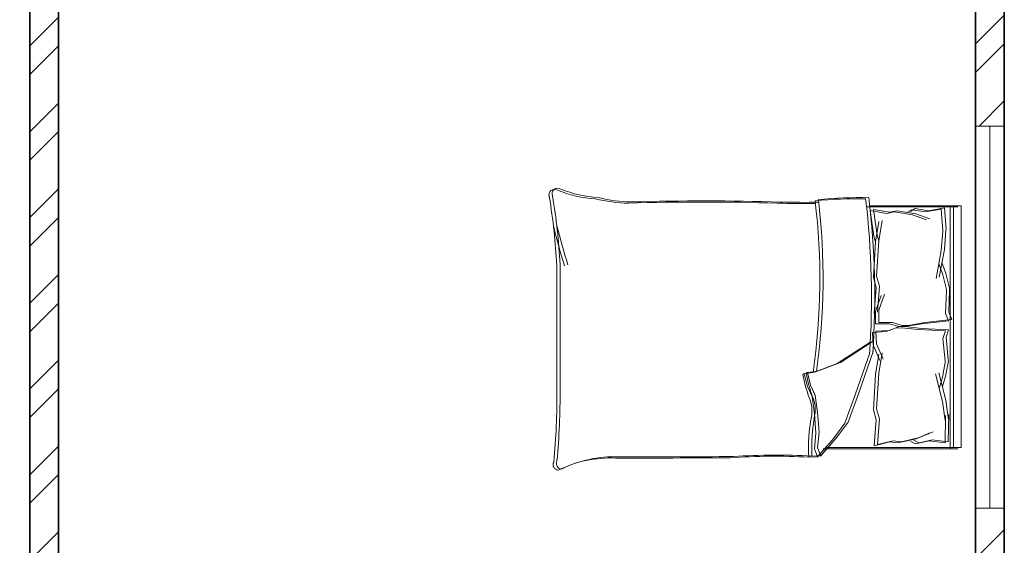
# Model space of a CAD drawing. Units: inches. Extents: x 1962 to 2771, y 1245 to 2660.
# Tile 13 of 114: x 2506 to 2661, y 1527 to 1609. Entities that reach past the tile are written whole.
import ezdxf

# ---------------------------------------------------------------- set-up
doc = ezdxf.new("R2010")
doc.units = ezdxf.units.IN
for name, color, linetype, lineweight in [('A-FURN', 8, 'Continuous', 13), ('A-GLAZ', 4, 'Continuous', 18), ('A-WALL', 7, 'Continuous', 35), ('A-WALL-PATT', 252, 'Continuous', 13)]:
    doc.layers.add(name, color=color, linetype=linetype, lineweight=lineweight)

# ---------------------------------------------------------------- blocks, each defined once
blk = doc.blocks.new('BED-PLAN')
for p, q in [((22.05, 42.03), (19.47, 39.08)), ((22.05, 42.02), (19.47, 39.08)), ((22.56, 42.21), (19.98, 39.26)), ((22.56, 42.21), (19.98, 39.26)), ((23.44, 42.09), (22.05, 42.03, 3.08)), ((23.44, 42.09), (22.05, 42.02, 3.08)), ((22.55, 40.8), (22.05, 42.03)), ((22.55, 40.8), (22.05, 42.02)), ((23.95, 42.27), (22.56, 42.21, 3.08)), ((23.95, 42.27), (22.56, 42.21, 3.08)), ((23.06, 40.98), (22.56, 42.21)), ((23.06, 40.98), (22.56, 42.21)), ((0, 40.75), (21.15, 40.75)), ((0, 40.75), (21.15, 40.75)), ((0, 2.76), (0, 40.75)), ((0.51, 40.93), (21.66, 40.93)), ((0.51, 40.93), (21.66, 40.93)), ((1.22, 2.76), (1.22, 40.75)), ((1.22, 2.76), (1.22, 40.75)), ((1.73, 2.95), (1.73, 40.93)), ((1.73, 2.95), (1.73, 40.93)), ((13.17, 40.3), (10.68, 39.68)), ((13.17, 40.3), (10.68, 39.68)), ((13.68, 40.48), (11.19, 39.87)), ((13.68, 40.48), (11.19, 39.87)), ((12.85, 36.22), (13.17, 40.3)), ((12.85, 36.22), (13.17, 40.3)), ((13.36, 36.4), (13.68, 40.48)), ((13.36, 36.4), (13.68, 40.48)), ((22.3, 38.34), (22.55, 40.8)), ((22.3, 38.34), (22.55, 40.8)), ((22.81, 38.52), (23.06, 40.98)), ((22.81, 38.52), (23.06, 40.98)), ((2.03, 39.83), (1.96, 35.54)), ((2.03, 39.83), (1.96, 35.54)), ((2.03, 39.83), (4.58, 39.53)), ((2.03, 39.83), (4.58, 39.53)), ((2.54, 40.02), (2.46, 35.72)), ((2.54, 40.02), (2.46, 35.72)), ((2.54, 40.02), (5.09, 39.72)), ((2.54, 40.02), (5.09, 39.72)), ((6.56, 39.2), (4.43, 38.26)), ((6.56, 39.2), (4.43, 38.26)), ((4.58, 39.53), (6.63, 40.01)), ((4.58, 39.53), (6.63, 40.01)), ((7.07, 39.38), (4.94, 38.44)), ((7.07, 39.38), (4.94, 38.44)), ((5.09, 39.72), (7.14, 40.19)), ((5.09, 39.72), (7.14, 40.19)), ((9.4, 39.83), (6.56, 39.2)), ((9.4, 39.83), (6.56, 39.2)), ((6.63, 40.01), (7.46, 39.6)), ((6.63, 40.01), (7.46, 39.6)), ((9.91, 40.02), (7.07, 39.38)), ((9.91, 40.02), (7.07, 39.38)), ((7.14, 40.19), (7.97, 39.78)), ((7.14, 40.19), (7.97, 39.78)), ((10.68, 39.68), (9.4, 39.83)), ((10.68, 39.68), (9.4, 39.83)), ((11.19, 39.87), (9.91, 40.02)), ((11.19, 39.87), (9.91, 40.02)), ((19.47, 39.08), (17.75, 36.74)), ((19.47, 39.08), (17.75, 36.74)), ((19.98, 39.26), (18.26, 36.92)), ((19.98, 39.26), (18.26, 36.92)), ((22.55, 35.26), (22.3, 38.34)), ((22.55, 35.26), (22.3, 38.34)), ((23.06, 35.45), (22.81, 38.52)), ((23.06, 35.44), (22.81, 38.52)), ((1.96, 35.54), (2.02, 36.34)), ((1.96, 35.54), (2.02, 36.34)), ((2.02, 36.34), (2.44, 33.32)), ((2.02, 36.34), (2.44, 33.32)), ((2.46, 35.72), (2.53, 36.52)), ((2.46, 35.72), (2.53, 36.52)), ((2.53, 36.52), (2.95, 33.5)), ((2.53, 36.52), (2.95, 33.5)), ((13.3, 34.66), (12.85, 36.22)), ((13.3, 34.66), (12.85, 36.22)), ((13.8, 34.84), (13.36, 36.4)), ((13.8, 34.84), (13.36, 36.4)), ((17.75, 36.74), (16.15, 32.31)), ((17.75, 36.74), (16.15, 32.31)), ((18.26, 36.92), (16.66, 32.49)), ((18.26, 36.92), (16.66, 32.49)), ((12.95, 29.09), (13.3, 34.66)), ((12.95, 29.09), (13.3, 34.66)), ((13.46, 29.27), (13.8, 34.84)), ((13.46, 29.27), (13.8, 34.84)), ((22.92, 32.56), (22.55, 35.26)), ((22.92, 32.55), (22.55, 35.26)), ((23.42, 32.74), (23.06, 35.45)), ((23.42, 32.74), (23.06, 35.44)), ((2.44, 33.32), (3.52, 29.01)), ((2.44, 33.32), (3.52, 29.01)), ((2.95, 33.5), (4.02, 29.19)), ((2.95, 33.5), (4.02, 29.19)), ((16.66, 32.49), (14.33, 25.86)), ((16.66, 32.49), (14.33, 25.86)), ((23.65, 30.95), (22.92, 32.56)), ((23.65, 30.95), (22.92, 32.55)), ((24.16, 31.14), (23.42, 32.74)), ((24.16, 31.14), (23.42, 32.74)), ((2.92, 31.16), (2.45, 29.52)), ((2.92, 31.16), (2.45, 29.52)), ((3.43, 31.34), (2.96, 29.7)), ((3.43, 31.34), (2.96, 29.7)), ((16.15, 32.31), (13.82, 25.68)), ((16.15, 32.31), (13.82, 25.68)), ((24.15, 28.99), (23.65, 30.95)), ((24.15, 28.98), (23.65, 30.95)), ((24.65, 29.17), (24.16, 31.14)), ((24.65, 29.17), (24.16, 31.14)), ((62.99, 11.98), (62.99, 31.54)), ((62.99, 11.97), (62.99, 31.54)), ((63.5, 12.16), (63.5, 31.72)), ((63.5, 12.16), (63.5, 31.72)), ((2.45, 29.52), (2.02, 27.19)), ((2.45, 29.52), (2.02, 27.19)), ((2.96, 29.7), (2.52, 27.37)), ((2.96, 29.7), (2.52, 27.37)), ((12.42, 25.89), (12.95, 29.09)), ((12.42, 25.89), (12.95, 29.09)), ((12.93, 26.07), (13.46, 29.27)), ((12.93, 26.07), (13.46, 29.27)), ((18.98, 27.38), (22.55, 28.74)), ((18.98, 27.38), (22.55, 28.74)), ((19.49, 27.57), (23.06, 28.92)), ((19.49, 27.57), (23.06, 28.92)), ((22.55, 28.74), (24.15, 28.99)), ((22.55, 28.74), (24.15, 28.98)), ((23.06, 28.92), (24.65, 29.17)), ((23.06, 28.92), (24.65, 29.17)), ((2.02, 27.19), (2.03, 26.94)), ((2.02, 27.19), (2.03, 26.93)), ((2.03, 26.94), (2.37, 23.42)), ((2.03, 26.93), (2.37, 23.42)), ((2.52, 27.37), (2.54, 27.12)), ((2.52, 27.37), (2.54, 27.12)), ((2.54, 27.12), (2.88, 23.6)), ((2.54, 27.12), (2.88, 23.6)), ((13.31, 24.44), (12.28, 26.89)), ((13.31, 24.44), (12.28, 26.88)), ((13.81, 24.63), (12.79, 27.07)), ((13.81, 24.63), (12.79, 27.07)), ((13.82, 24.05), (18.98, 27.38)), ((13.82, 24.05), (18.98, 27.38)), ((14.33, 24.24), (19.49, 27.57)), ((14.33, 24.24), (19.49, 27.57)), ((2.37, 23.42), (1.98, 22.24)), ((2.37, 23.42), (1.98, 22.24)), ((2.88, 23.6), (2.49, 22.42)), ((2.88, 23.6), (2.49, 22.42)), ((13.43, 22.49), (13.31, 24.44)), ((13.43, 22.49), (13.31, 24.44)), ((13.94, 22.68), (13.81, 24.63)), ((13.94, 22.68), (13.81, 24.63)), ((1.98, 22.24), (6.25, 22.05)), ((1.98, 22.24), (6.25, 22.05)), ((2.49, 22.42), (6.76, 22.23)), ((2.49, 22.42), (6.76, 22.23)), ((6.25, 22.05), (8.81, 21.75)), ((6.25, 22.05), (8.81, 21.75)), ((6.25, 21.3), (8.78, 21.76)), ((6.25, 21.3), (8.78, 21.76)), ((6.76, 22.23), (9.31, 21.93)), ((6.76, 22.23), (9.31, 21.93)), ((8.78, 21.76), (9.81, 21.76)), ((8.78, 21.76), (9.81, 21.76)), ((8.81, 21.75), (9.84, 21.81)), ((8.81, 21.75), (9.84, 21.81)), ((9.31, 21.93), (10.35, 21.99)), ((9.31, 21.93), (10.35, 21.99)), ((9.81, 21.76), (11.3, 21.3)), ((9.81, 21.76), (11.3, 21.3)), ((9.84, 21.81), (11.3, 22.36)), ((9.84, 21.81), (11.3, 22.36)), ((10.35, 21.99), (11.81, 22.54)), ((10.35, 21.99), (11.81, 22.54)), ((11.3, 22.36), (13.43, 22.49)), ((11.3, 22.36), (13.43, 22.49)), ((11.81, 22.54), (13.94, 22.68)), ((11.81, 22.54), (13.94, 22.68)), ((1.49, 20.65), (5.74, 21.11)), ((1.49, 20.65), (5.74, 21.11)), ((1.95, 19.51), (1.49, 20.65)), ((1.95, 19.51), (1.49, 20.65)), ((1.99, 20.84), (6.25, 21.3)), ((1.99, 20.84), (6.25, 21.3)), ((2.45, 19.69), (1.99, 20.84)), ((2.45, 19.69), (1.99, 20.84)), ((5.74, 21.11), (8.27, 21.57)), ((5.74, 21.11), (8.27, 21.57)), ((8.27, 21.57), (9.3, 21.57)), ((8.27, 21.57), (9.3, 21.57)), ((9.3, 21.57), (10.8, 21.11)), ((9.3, 21.57), (10.8, 21.11)), ((10.8, 21.11), (12.93, 21.11)), ((10.8, 21.11), (12.93, 21.11)), ((11.3, 21.3), (13.44, 21.3)), ((11.3, 21.3), (13.44, 21.3)), ((12.93, 21.11), (12.93, 19.16)), ((12.93, 21.11), (12.93, 19.16)), ((13.44, 21.3), (13.44, 19.34)), ((13.44, 21.3), (13.44, 19.34)), ((1.83, 15.97), (1.95, 19.51)), ((1.83, 15.97), (1.95, 19.51)), ((2.34, 16.15), (2.45, 19.69)), ((2.34, 16.15), (2.45, 19.69)), ((12.93, 19.16), (12.06, 16.66)), ((12.93, 19.16), (12.06, 16.66)), ((13.44, 19.34), (12.57, 16.84)), ((13.44, 19.34), (12.57, 16.84)), ((12.85, 15.41), (13.17, 19.49)), ((12.85, 15.41), (13.17, 19.49)), ((13.36, 15.59), (13.68, 19.67)), ((13.36, 15.59), (13.68, 19.67)), ((1.83, 15.72), (1.83, 15.97)), ((1.83, 15.72), (1.83, 15.97)), ((2.41, 13.42), (1.83, 15.72)), ((2.41, 13.42), (1.83, 15.72)), ((2.34, 15.9), (2.34, 16.15)), ((2.34, 15.9), (2.34, 16.15)), ((2.91, 13.6), (2.34, 15.9)), ((2.91, 13.6), (2.34, 15.9)), ((13.8, 14.03), (13.36, 15.59)), ((13.8, 14.03), (13.36, 15.59)), ((2.64, 9.63), (3.44, 13.99)), ((2.64, 9.63), (3.44, 13.99)), ((3.14, 9.81), (3.95, 14.17)), ((3.14, 9.81), (3.95, 14.17)), ((13.3, 13.85), (12.85, 15.41)), ((13.3, 13.85), (12.85, 15.41)), ((13.46, 8.46), (13.8, 14.03)), ((13.46, 8.46), (13.8, 14.03)), ((2.98, 11.81), (2.41, 13.42)), ((2.98, 11.81), (2.41, 13.42)), ((3.49, 11.99), (2.91, 13.6)), ((3.49, 11.99), (2.91, 13.6)), ((12.95, 8.28), (13.3, 13.85)), ((12.95, 8.28), (13.3, 13.85)), ((2.41, 6.59), (2.64, 9.63)), ((2.41, 6.59), (2.64, 9.63)), ((2.91, 6.77), (3.14, 9.81)), ((2.91, 6.77), (3.14, 9.81)), ((12.42, 5.07), (12.95, 8.28)), ((12.42, 5.07), (12.95, 8.28)), ((12.93, 5.26), (13.46, 8.46)), ((12.93, 5.26), (13.46, 8.46)), ((12.95, 8.28), (13.21, 7.38)), ((12.95, 8.28), (13.21, 7.38)), ((13.46, 8.46), (13.72, 7.56)), ((13.46, 8.46), (13.72, 7.56)), ((2.39, 6.5), (2.41, 6.59)), ((2.39, 6.5), (2.41, 6.59)), ((2.65, 3.1), (2.39, 6.5)), ((2.65, 3.1), (2.39, 6.5)), ((2.9, 6.68), (2.91, 6.77)), ((2.9, 6.68), (2.91, 6.77)), ((3.16, 3.28), (2.9, 6.68)), ((3.16, 3.28), (2.9, 6.68)), ((13.21, 7.38), (13.78, 3.33)), ((13.21, 7.38), (13.78, 3.33)), ((13.72, 7.56), (14.29, 3.51)), ((13.72, 7.56), (14.29, 3.51)), ((7.12, 4.02), (4.93, 4.82)), ((7.12, 4.02), (4.93, 4.82)), ((7.63, 4.2), (5.44, 5)), ((7.63, 4.2), (5.44, 5)), ((2.64, 3.1), (5.16, 3.56)), ((2.64, 3.1), (5.16, 3.56)), ((3.14, 3.28), (5.67, 3.74)), ((3.14, 3.28), (5.67, 3.74)), ((5.16, 3.56), (7.23, 3.21)), ((5.16, 3.56), (7.23, 3.21)), ((5.67, 3.74), (7.74, 3.39)), ((5.67, 3.74), (7.74, 3.39)), ((9.99, 3.56), (7.12, 4.02)), ((9.99, 3.56), (7.12, 4.02)), ((7.23, 3.21), (8.04, 3.67)), ((7.23, 3.21), (8.04, 3.67)), ((10.5, 3.74), (7.63, 4.2)), ((10.5, 3.74), (7.63, 4.2)), ((7.74, 3.39), (8.55, 3.85)), ((7.74, 3.39), (8.55, 3.85)), ((11.26, 3.79), (9.99, 3.56)), ((11.26, 3.79), (9.99, 3.56)), ((11.76, 3.97), (10.5, 3.74)), ((11.76, 3.97), (10.5, 3.74)), ((13.78, 3.33), (11.26, 3.79)), ((13.78, 3.33), (11.26, 3.79)), ((14.29, 3.51), (11.76, 3.97)), ((14.29, 3.51), (11.76, 3.97)), ((14.4, 2.76), (0, 2.76)), ((14.4, 2.76), (0, 2.76)), ((14.9, 2.95), (0.51, 2.95)), ((14.9, 2.95), (0.51, 2.95))]:
    blk.add_line(p, q)
for centre, radius, start, end in [((54.58, 60.54), 18.33, 267.4714, 296.4681), ((54.58, 60.54), 18.33, 267.4714, 296.4681), ((55.09, 60.72), 18.33, 267.4714, 296.4681), ((55.09, 60.72), 18.33, 267.4714, 296.4681), ((62.69, 43.25), 0.876, 332.6588, 86.02), ((62.69, 43.25), 0.876, 332.6588, 86.02), ((63.2, 43.43), 0.876, 332.6588, 86.02), ((63.2, 43.43), 0.876, 332.6588, 86.02), ((-5.29, 40.8), 28.76, 349.8763, 2.5657), ((-5.29, 40.8), 28.76, 349.8763, 2.5657), ((28.87, 144.88), 102.94, 266.9791, 273.8365), ((28.87, 144.88), 102.94, 266.9791, 273.8365), ((-4.78, 40.98), 28.76, 349.8763, 2.5657), ((-4.78, 40.98), 28.76, 349.8763, 2.5657), ((29.37, 145.06), 102.94, 266.9791, 273.8365), ((29.37, 145.06), 102.94, 266.9791, 273.8365), ((53.91, -3583.94), 3626.16, 90.00217, 90.28689), ((53.91, -3583.94), 3626.16, 90.00217, 90.28689), ((54.42, -3583.75), 3626.16, 90.00217, 90.28689), ((54.42, -3583.75), 3626.16, 90.00217, 90.28689), ((168.74, 32.71), 105.75, 174.4998, 180.6351), ((168.74, 32.71), 105.75, 174.4998, 180.6351), ((169.24, 32.89), 105.75, 174.4998, 180.6351), ((169.24, 32.89), 105.75, 174.4998, 180.6351), ((27.87, 34.77), 4.95, 168.6608, 203.7384), ((27.87, 34.77), 4.95, 168.6608, 203.7384), ((28.38, 34.95), 4.95, 168.6608, 203.7384), ((28.38, 34.95), 4.95, 168.6608, 203.7384), ((1.18, 24.77), 23.57, 10.6617, 19.8806), ((1.18, 24.76), 23.57, 10.6617, 19.8806), ((1.69, 24.95), 23.57, 10.6617, 19.8806), ((1.69, 24.95), 23.57, 10.6617, 19.8806), ((124.25, 14.12), 102.56, 171.7845, 186.9006), ((124.25, 14.11), 102.56, 171.7845, 186.9006), ((124.76, 14.3), 102.56, 171.7845, 186.9006), ((124.76, 14.3), 102.56, 171.7845, 186.9006), ((24.2, 29.12), 0.147, 250.2464, 1.1377), ((24.2, 29.12), 0.147, 250.2464, 1.1377), ((24.7, 29.3), 0.147, 250.2464, 1.1377), ((24.7, 29.3), 0.147, 250.2464, 1.1377), ((144.71, 16.98), 131.13, 176.0865, 186.7821), ((144.71, 16.98), 131.13, 176.0865, 186.7821), ((145.22, 17.16), 131.13, 176.0865, 186.7821), ((145.22, 17.16), 131.13, 176.0865, 186.7821), ((-18.85, -13.69), 84.62, 13.3832, 17.7053), ((-18.85, -13.69), 84.62, 13.3832, 17.7053), ((-18.34, -13.51), 84.62, 13.3832, 17.7053), ((-18.34, -13.51), 84.62, 13.3832, 17.7053), ((159.64, 17.03), 96.78, 182.9958, 189.4091), ((159.64, 17.03), 96.78, 182.9958, 189.4091), ((160.15, 17.21), 96.78, 182.9958, 189.4091), ((160.15, 17.21), 96.78, 182.9958, 189.4091), ((15.97, 67.7), 66.22, 268.7218, 275.604), ((15.97, 67.7), 66.22, 268.7218, 275.604), ((16.48, 67.88), 66.22, 268.7218, 275.604), ((16.48, 67.88), 66.22, 268.7218, 275.604), ((24.78, -132.99), 135.22, 88.4762, 91.0082), ((24.78, -132.99), 135.22, 88.4762, 91.0082), ((25.29, -132.81), 135.22, 88.4762, 91.0082), ((25.29, -132.81), 135.22, 88.4762, 91.0082), ((40.23, 385.38), 383.38, 268.2277, 271.7185), ((40.23, 385.38), 383.38, 268.2277, 271.7185), ((40.74, 385.56), 383.38, 268.2277, 271.7185), ((40.74, 385.56), 383.38, 268.2277, 271.7185), ((51.28, -21.38), 23.56, 76.0648, 88.9113), ((51.28, -21.38), 23.56, 76.0648, 88.9113), ((51.79, -21.2), 23.56, 76.0648, 88.9113), ((51.79, -21.2), 23.56, 76.0648, 88.9113), ((56.37, -17.03), 18.73, 67.9751, 86.652), ((56.37, -17.03), 18.73, 67.9751, 86.652), ((55.86, -17.22), 18.73, 67.9751, 86.652), ((55.86, -17.22), 18.73, 67.9751, 86.652), ((63.37, 0.87), 0.866, 236.1736, 23.4781), ((63.37, 0.87), 0.866, 236.1736, 23.4781), ((63.87, 1.05), 0.866, 236.1736, 23.4781), ((63.87, 1.05), 0.866, 236.1736, 23.4781)]:
    blk.add_arc(centre, radius, start, end)
blk = doc.blocks.new('WIN-60IN-A')
for p, q in [((0, 60), (4.5, 60)), ((4.5, 60), (2.25, 60)), ((2.25, 60), (2.25, 0)), ((2.25, 0), (0, 0)), ((0, 0), (4.5, 0))]:
    blk.add_line(p, q)

msp = doc.modelspace()

# ---------------------------------------------------------------- hatches: boundary and pattern name
at = {"layer": 'A-WALL-PATT'}
h = msp.add_hatch(dxfattribs=at)
h.set_pattern_fill('ANSI32', color=256)
h.paths.add_polyline_path([(2090.8074, 2467.3437), (2141.6481, 2467.3437), (2141.6481, 2469.5937), (2141.6481, 2471.8437), (2086.3074, 2471.8437), (2086.3074, 2422.5333), (2090.8074, 2422.5333)])
h.paths.add_polyline_path([(2282.7664, 2471.8437), (2204.8982, 2471.8437), (2204.8982, 2467.3437), (2234.8074, 2467.3437), (2234.8074, 2311.3437), (2228.7492, 2311.3437), (2228.7492, 2306.8437), (2234.8074, 2306.8437), (2331.9227, 2306.8437), (2331.9227, 2309.0937), (2331.9227, 2311.3437), (2239.3074, 2311.3437), (2239.3074, 2467.3437), (2282.7664, 2467.3437), (2282.7664, 2469.5937)])
h.paths.add_polyline_path([(2471.4531, 2519.8437), (2552.011, 2519.8437), (2564.3996, 2519.8437), (2564.3996, 2511.1389), (2568.8996, 2511.1389), (2568.8996, 2524.3437), (2466.9531, 2524.3437), (2466.9531, 2471.8437), (2450.0749, 2471.8437), (2446.4672, 2471.8437), (2446.4672, 2467.3437), (2450.0749, 2467.3437), (2475.9988, 2467.3437), (2475.9988, 2469.5937), (2475.9988, 2471.8437), (2471.4531, 2471.8437)])
h.paths.add_polyline_path([(2575.2231, 2469.5937), (2575.2231, 2471.8437), (2568.8996, 2471.8437), (2568.8996, 2487.1389), (2564.3996, 2487.1389), (2564.3996, 2471.8437), (2556.511, 2471.8437), (2499.2904, 2471.8437), (2499.2904, 2467.3437), (2507.8074, 2467.3437), (2507.8074, 2311.3437), (2414.863, 2311.3437), (2414.863, 2306.8437), (2512.3074, 2306.8437), (2517.0114, 2306.8437), (2517.0114, 2309.0937), (2517.0114, 2311.3437), (2512.3074, 2311.3437), (2512.3074, 2467.3437), (2575.2231, 2467.3437)])
h.paths.add_polyline_path([(2660.8074, 2471.8437), (2600.9602, 2471.8437), (2600.9602, 2467.3437), (2656.3074, 2467.3437), (2656.3074, 2432.5704), (2660.8074, 2432.5704)])
h.paths.add_polyline_path([(2660.8074, 2372.5704), (2656.3074, 2372.5704), (2656.3074, 2311.3437), (2600.276, 2311.3437), (2600.276, 2309.0937), (2600.276, 2306.8437), (2656.3074, 2306.8437), (2656.3074, 2296.2593), (2660.8074, 2296.2593)])
h.paths.add_polyline_path([(2572.3074, 2306.8437), (2577.1385, 2306.8437), (2577.1385, 2311.3437), (2551.082, 2311.3437), (2551.082, 2306.8437), (2567.8074, 2306.8437), (2567.8074, 2258.8437), (2540.0574, 2258.8437), (2540.0574, 2256.5937), (2540.0574, 2254.3437), (2567.8074, 2254.3437), (2656.3074, 2254.3437), (2656.3074, 2236.9085), (2660.8074, 2236.9085), (2660.8074, 2272.2593), (2656.3074, 2272.2593), (2656.3074, 2258.8437), (2572.3074, 2258.8437)])
h.paths.add_polyline_path([(2512.3074, 2254.3437), (2518.8716, 2254.3437), (2518.8716, 2256.5937), (2518.8716, 2258.8437), (2507.8074, 2258.8437), (2507.8074, 2177.8437), (2567.8074, 2177.8437), (2567.8074, 2172.9628), (2572.3074, 2172.9628), (2572.3074, 2177.8437), (2656.3074, 2177.8437), (2656.3074, 2166.4846), (2660.8074, 2166.4846), (2660.8074, 2200.9085), (2656.3074, 2200.9085), (2656.3074, 2182.3437), (2512.3074, 2182.3437)])
h.paths.add_polyline_path([(2656.3074, 2129.8437), (2572.3074, 2129.8437), (2572.3074, 2150.3044), (2570.0574, 2150.3044), (2567.8074, 2150.3044), (2567.8074, 2129.8437), (2507.8074, 2129.8437), (2507.8074, 2116.3027), (2510.0574, 2116.3027), (2512.3074, 2116.3027), (2512.3074, 2125.3437), (2567.8074, 2125.3437), (2572.3074, 2125.3437), (2656.3074, 2125.3437)])
h.paths.add_polyline_path([(2090.8074, 2362.5333), (2086.3074, 2362.5333), (2086.3074, 2298.6242), (2090.8074, 2298.6242), (2090.8074, 2306.8437), (2174.8074, 2306.8437), (2174.8074, 2286.4178), (2179.3074, 2286.4178), (2179.3074, 2306.8437), (2192.8641, 2306.8437), (2192.8641, 2309.0937), (2192.8641, 2311.3437), (2090.8074, 2311.3437)])
h.paths.add_polyline_path([(2209.156, 2258.8437), (2179.3074, 2258.8437), (2179.3074, 2263.2236), (2177.0574, 2263.2236), (2174.8074, 2263.2236), (2174.8074, 2258.8437), (2090.8074, 2258.8437), (2090.8074, 2274.6242), (2086.3074, 2274.6242), (2086.3074, 2238.2967), (2088.5574, 2238.2967), (2090.8074, 2238.2967), (2090.8074, 2254.3437), (2209.156, 2254.3437)])
h.paths.add_polyline_path([(2090.8074, 2177.8437), (2234.8074, 2177.8437), (2234.8074, 2173.1428), (2239.3074, 2173.1428), (2239.3074, 2258.8437), (2230.8442, 2258.8437), (2230.8442, 2256.5937), (2230.8442, 2254.3437), (2234.8074, 2254.3437), (2234.8074, 2182.3437), (2090.8074, 2182.3437), (2090.8074, 2202.2967), (2086.3074, 2202.2967), (2086.3074, 2140.0389), (2090.8074, 2140.0389)])
h.paths.add_polyline_path([(2090.8074, 2080.0389), (2086.3074, 2080.0389), (2086.3074, 2033.8437), (2090.8074, 2033.8437)], flags=17)
h.paths.add_polyline_path([(2244.9405, 2033.8437), (2239.3074, 2033.8437), (2239.3074, 2142.0665), (2237.2592, 2142.0665), (2234.8074, 2142.0665), (2234.8074, 2033.8437), (2090.8074, 2033.8437), (2076.5204, 2033.8437), (2072.0204, 2033.8437), (2072.0204, 2000.4493), (2076.5204, 2000.4493), (2076.5204, 2029.3437), (2090.8074, 2029.3437), (2244.9405, 2029.3437), (2244.9405, 2031.5937)])
h.paths.add_polyline_path([(2234.8074, 1933.3437), (2076.5204, 1933.3437), (2076.5204, 1952.4493), (2074.2704, 1952.4493), (2072.0204, 1952.4493), (2072.0204, 1933.3437), (2072.0204, 1928.8437), (2234.8074, 1928.8437)])
h.paths.add_polyline_path([(2090.8074, 1928.8437), (2086.3074, 1928.8437), (2086.3074, 1906.5013), (2090.8074, 1906.5013)])
h.paths.add_polyline_path([(2090.8074, 1846.5013), (2086.3074, 1846.5013), (2086.3074, 1769.9917), (2088.5574, 1769.9917), (2090.8074, 1769.9917), (2090.8074, 1780.3437), (2234.8074, 1780.3437), (2234.8074, 1708.3437), (2230.3764, 1708.3437), (2230.3764, 1703.8437), (2239.3074, 1703.8437), (2239.3074, 1792.6669), (2237.0574, 1792.6669), (2234.8074, 1792.6669), (2234.8074, 1784.8437), (2090.8074, 1784.8437)])
h.paths.add_polyline_path([(2239.3074, 1928.8437), (2244.9405, 1928.8437), (2244.9405, 1931.0937), (2244.9405, 1933.3437), (2234.8074, 1933.3437), (2234.8074, 1928.8437), (2234.8074, 1825.5949), (2239.3074, 1825.5949)])
h.paths.add_polyline_path([(2148.0425, 1649.0937), (2148.0425, 1651.3437), (2090.8074, 1651.3437), (2090.8074, 1646.8437), (2148.0425, 1646.8437)], flags=0)
h.paths.add_polyline_path([(2207.5601, 1708.3437), (2090.8074, 1708.3437), (2090.8074, 1703.8437), (2174.8074, 1703.8437), (2174.8074, 1651.3437), (2170.4457, 1651.3437), (2170.4457, 1646.8437), (2195.9924, 1646.8437), (2195.9924, 1649.0937), (2195.9924, 1651.3437), (2179.3074, 1651.3437), (2179.3074, 1703.8437), (2207.5601, 1703.8437), (2207.5601, 1706.0937)])
h.paths.add_polyline_path([(2090.8074, 1733.9917), (2086.3074, 1733.9917), (2086.3074, 1696.1032), (2088.5574, 1696.1032), (2090.8074, 1696.1032)])
h.paths.add_polyline_path([(2090.8074, 1672.1032), (2086.3074, 1672.1032), (2086.3074, 1600.3335), (2090.8074, 1600.3335)])
h.paths.add_polyline_path([(2090.8074, 1540.3335), (2086.3074, 1540.3335), (2086.3074, 1486.3437), (2139.6766, 1486.3437), (2139.6766, 1490.8437), (2090.8074, 1490.8437)])
h.paths.add_polyline_path([(2302.3876, 1490.8437), (2239.3074, 1490.8437), (2239.3074, 1646.8437), (2335.9994, 1646.8437), (2335.9994, 1651.3437), (2229.884, 1651.3437), (2229.884, 1646.8437), (2234.8074, 1646.8437), (2234.8074, 1490.8437), (2202.7103, 1490.8437), (2202.7103, 1488.5937), (2202.7103, 1486.3437), (2275.0699, 1486.3437), (2275.0699, 1475.772), (2279.5699, 1475.772), (2279.5699, 1486.3437), (2302.3876, 1486.3437)])
h.paths.add_polyline_path([(2279.5699, 1451.772), (2275.0699, 1451.772), (2275.0699, 1438.3437), (2174.8074, 1438.3437), (2174.8074, 1486.3437), (2179.7922, 1486.3437), (2179.7922, 1490.8437), (2163.3585, 1490.8437), (2163.3585, 1488.5937), (2163.3585, 1486.3437), (2170.3074, 1486.3437), (2170.3074, 1433.8437), (2279.5699, 1433.8437)])
h.paths.add_polyline_path([(2427.2363, 1490.8437), (2375.8074, 1490.8437), (2375.8074, 1646.8437), (2381.6401, 1646.8437), (2381.6401, 1651.3437), (2365.887, 1651.3437), (2365.887, 1649.0937), (2365.887, 1646.8437), (2371.3074, 1646.8437), (2371.3074, 1490.8437), (2327.5627, 1490.8437), (2327.5627, 1488.5937), (2327.5627, 1486.3437), (2371.3074, 1486.3437), (2371.3074, 1433.8437), (2375.8074, 1433.8437), (2375.8074, 1486.3437), (2427.2363, 1486.3437)])
h.paths.add_polyline_path([(2512.3074, 1646.8437), (2519.4351, 1646.8437), (2519.4351, 1649.0937), (2519.4351, 1651.3437), (2507.8074, 1651.3437), (2416.0063, 1651.3437), (2416.0063, 1649.0937), (2416.0063, 1646.8437), (2507.8074, 1646.8437), (2507.8074, 1490.8437), (2497.0532, 1490.8437), (2497.0532, 1488.5937), (2497.0532, 1486.3437), (2574.9344, 1486.3437), (2574.9344, 1476.0181), (2579.4344, 1476.0181), (2579.4344, 1486.3437), (2584.4872, 1486.3437), (2584.3074, 1490.8437), (2512.3074, 1490.8437)])
h.paths.add_polyline_path([(2470.5091, 1486.3437), (2473.9767, 1486.3437), (2473.9767, 1490.8437), (2449.6605, 1490.8437), (2449.6605, 1488.5937), (2449.6605, 1486.3437), (2466.0091, 1486.3437), (2466.0091, 1433.8437), (2470.5091, 1433.8437), (2579.4344, 1433.8437), (2579.4344, 1452.0181), (2574.9344, 1452.0181), (2574.9344, 1438.3437), (2554.5091, 1438.3437), (2470.5091, 1438.3437)])
h.paths.add_polyline_path([(2656.3074, 1490.8437), (2611.86, 1490.8437), (2611.86, 1486.3437), (2656.3074, 1486.3437)])
h.paths.add_polyline_path([(2660.8074, 1532.7007), (2658.5574, 1532.7007), (2656.3074, 1532.7007), (2656.3074, 1486.3437), (2660.8074, 1486.3437)])
h.paths.add_polyline_path([(2660.8074, 1664.9663), (2656.3074, 1664.9663), (2656.3074, 1651.3437), (2602.2313, 1651.3437), (2602.2313, 1646.8437), (2656.3074, 1646.8437), (2656.3074, 1592.7007), (2660.8074, 1592.7007)])
h.paths.add_polyline_path([(2660.8074, 1724.5221), (2656.3074, 1724.5221), (2656.3074, 1703.8437), (2542.4725, 1703.8437), (2542.4725, 1699.3437), (2567.8074, 1699.3437), (2567.8074, 1651.3437), (2552.7766, 1651.3437), (2552.7766, 1649.0937), (2552.7766, 1646.8437), (2577.2878, 1646.8437), (2577.2878, 1649.0937), (2577.2878, 1651.3437), (2572.3074, 1651.3437), (2572.3074, 1699.3437), (2656.3074, 1699.3437), (2656.3074, 1688.9663), (2660.8074, 1688.9663)])
h.paths.add_polyline_path([(2660.8074, 1880.6524), (2656.3074, 1880.6524), (2656.3074, 1832.8437), (2512.3074, 1832.8437), (2512.3074, 1837.8959), (2507.8074, 1837.8959), (2507.8074, 1828.3437), (2567.8074, 1828.3437), (2567.8074, 1804.3437), (2572.3074, 1804.3437), (2572.3074, 1828.3437), (2656.3074, 1828.3437), (2656.3074, 1818.6778), (2660.8074, 1818.6778)])
h.paths.add_polyline_path([(2660.8074, 1794.6778), (2656.3074, 1794.6778), (2656.3074, 1780.3437), (2572.3074, 1780.3437), (2572.3074, 1783.0303), (2570.0574, 1783.0303), (2567.8074, 1783.0303), (2567.8074, 1780.3437), (2507.8074, 1780.3437), (2507.8074, 1699.3437), (2517.8858, 1699.3437), (2517.8858, 1701.5937), (2517.8858, 1703.8437), (2512.3074, 1703.8437), (2512.3074, 1775.8437), (2656.3074, 1775.8437), (2656.3074, 1760.5221), (2660.8074, 1760.5221)])
h.paths.add_polyline_path([(2660.8074, 1981.3437), (2660.8074, 2020.2808), (2658.5574, 2020.2808), (2656.3074, 2020.2808), (2656.3074, 1981.3437), (2512.3074, 1981.3437), (2512.3074, 2086.6996), (2507.8074, 2086.6996), (2507.8074, 1981.3437), (2375.8074, 1981.3437), (2375.8074, 1986.8505), (2373.5574, 1986.8505), (2371.3074, 1986.8505), (2371.3074, 1973.2607), (2375.8074, 1973.2607), (2375.8074, 1976.8437), (2507.8074, 1976.8437), (2507.8074, 1865.4281), (2510.0574, 1865.4281), (2512.3074, 1865.4281), (2512.3074, 1976.8437), (2660.8074, 1976.8437)])
h.paths.add_polyline_path([(2375.8074, 1940.297), (2373.5574, 1940.297), (2371.3074, 1940.297), (2371.3074, 1933.3437), (2278.4434, 1933.3437), (2278.4434, 1928.8437), (2371.3074, 1928.8437), (2371.3074, 1651.3437), (2375.8074, 1651.3437)])
h.paths.add_polyline_path([(2660.8074, 1976.8437), (2656.3074, 1976.8437), (2656.3074, 1940.6524), (2660.8074, 1940.6524)], flags=17)
h.paths.add_polyline_path([(2660.8074, 2142.4846), (2656.3074, 2142.4846), (2656.3074, 2080.2808), (2660.8074, 2080.2808)])
h.paths.add_polyline_path([(2381.4189, 2311.3437), (2375.8074, 2311.3437), (2375.8074, 2467.3437), (2424.7242, 2467.3437), (2424.7242, 2469.5937), (2424.7242, 2471.8437), (2375.8074, 2471.8437), (2375.8074, 2524.3437), (2371.3074, 2524.3437), (2371.3074, 2471.8437), (2307.2097, 2471.8437), (2307.2097, 2467.3437), (2371.3074, 2467.3437), (2371.3074, 2311.3437), (2366.8901, 2311.3437), (2366.8901, 2306.8437), (2371.3074, 2306.8437), (2371.3074, 2033.8437), (2279.6589, 2033.8437), (2279.6589, 2029.3437), (2371.3074, 2029.3437), (2371.3074, 2014.2598), (2375.8074, 2014.2598), (2375.8074, 2306.8437), (2381.4189, 2306.8437)])
h.paths.add_polyline_path([(2263.3074, 2524.3437), (2170.3074, 2524.3437), (2170.3074, 2519.8437), (2170.3074, 2471.8437), (2165.0312, 2471.8437), (2165.0312, 2467.3437), (2179.6721, 2467.3437), (2179.6721, 2469.5161), (2179.6721, 2471.8437), (2174.8074, 2471.8437), (2174.8074, 2519.8437), (2258.8074, 2519.8437), (2258.8074, 2511.6436), (2263.3074, 2511.6436)])
h.paths.add_polyline_path([(2245.0232, 1361.4123), (2492.9468, 1361.4123), (2492.9468, 1398.505), (2245.0232, 1398.505)], flags=9)
h.paths.add_polyline_path([(2388.1434, 2086.6936), (2425.0704, 2086.6936), (2425.0704, 2105.3509), (2388.1434, 2105.3509)], flags=9)
h.paths.add_polyline_path([(2404.922, 2242.6744), (2445.7337, 2242.6744), (2445.7337, 2261.3318), (2404.922, 2261.3318)], flags=9)
h.paths.add_polyline_path([(2269.4107, 2156.7935), (2306.3378, 2156.7935), (2306.3378, 2175.4508), (2269.4107, 2175.4508)], flags=9)
h.paths.add_polyline_path([(2269.3277, 2233.4343), (2306.2547, 2233.4343), (2306.2547, 2252.0917), (2269.3277, 2252.0917)], flags=9)
h.paths.add_polyline_path([(2431.6052, 2320.6922), (2470.4456, 2320.6922), (2470.4456, 2339.3495), (2431.6052, 2339.3495)], flags=25)
h.paths.add_polyline_path([(2249.6902, 2315.7608), (2288.5306, 2315.7608), (2288.5306, 2334.4182), (2249.6902, 2334.4182)], flags=25)
h.paths.add_polyline_path([(2096.9301, 2314.3181), (2135.7704, 2314.3181), (2135.7704, 2332.9755), (2096.9301, 2332.9755)], flags=25)
h.paths.add_polyline_path([(2134.3475, 2285.7089), (2161.4655, 2285.7089), (2161.4655, 2304.3662), (2134.3475, 2304.3662)], flags=9)
h.paths.add_polyline_path([(2126.5155, 2209.4076), (2159.9227, 2209.4076), (2159.9227, 2228.065), (2126.5155, 2228.065)], flags=25)
h.paths.add_polyline_path([(2110.5753, 2141.5299), (2149.4157, 2141.5299), (2149.4157, 2160.1872), (2110.5753, 2160.1872)], flags=25)
h.paths.add_polyline_path([(2249.8618, 1968.3317), (2286.3966, 1968.3317), (2286.3966, 1986.989), (2249.8618, 1986.989)], flags=9)
h.paths.add_polyline_path([(2395.9507, 1777.0051), (2436.7624, 1777.0051), (2436.7624, 1795.6625), (2395.9507, 1795.6625)], flags=9)
h.paths.add_polyline_path([(2398.5259, 1888.5651), (2435.0062, 1888.5651), (2435.0062, 1907.2224), (2398.5259, 1907.2224)], flags=25)
h.paths.add_polyline_path([(2259.3506, 1728.3559), (2296.2776, 1728.3559), (2296.2776, 1747.0132), (2259.3506, 1747.0132)], flags=9)
h.paths.add_polyline_path([(2271.3698, 1845.268), (2308.2968, 1845.268), (2308.2968, 1863.9253), (2271.3698, 1863.9253)], flags=9)
h.paths.add_polyline_path([(2120.9355, 1786.3027), (2159.7759, 1786.3027), (2159.7759, 1804.9601), (2120.9355, 1804.9601)], flags=25)
h.paths.add_polyline_path([(2121.3164, 1732.1043), (2154.7236, 1732.1043), (2154.7236, 1750.7616), (2121.3164, 1750.7616)], flags=25)
h.paths.add_polyline_path([(2118.3706, 1678.8997), (2147.5282, 1678.8997), (2147.5282, 1697.557), (2118.3706, 1697.557)], flags=25)
h.paths.add_polyline_path([(2385.9227, 1493.557), (2424.763, 1493.557), (2424.763, 1512.2143), (2385.9227, 1512.2143)], flags=25)
h.paths.add_polyline_path([(2248.7058, 1500.0256), (2287.5462, 1500.0256), (2287.5462, 1518.6829), (2248.7058, 1518.6829)], flags=25)
h.paths.add_polyline_path([(2104.1669, 1617.3771), (2143.0073, 1617.3771), (2143.0073, 1636.0344), (2104.1669, 1636.0344)], flags=9)
h.paths.add_polyline_path([(2096.0714, 1447.8824), (2137.3845, 1447.8824), (2137.3845, 1458.1859), (2096.0714, 1458.1859)], flags=9)
h.paths.add_polyline_path([(2180.6114, 1440.325), (2209.7689, 1440.325), (2209.7689, 1458.9823), (2180.6114, 1458.9823)], flags=25)
h.paths.add_polyline_path([(2316.1698, 1447.9637), (2357.4829, 1447.9637), (2357.4829, 1458.2673), (2316.1698, 1458.2673)], flags=9)
h.paths.add_polyline_path([(2397.6187, 1447.9637), (2438.9318, 1447.9637), (2438.9318, 1458.2673), (2397.6187, 1458.2673)], flags=9)
h.paths.add_polyline_path([(2473.0778, 1439.5953), (2502.2354, 1439.5953), (2502.2354, 1458.2527), (2473.0778, 1458.2527)], flags=25)
h.paths.add_polyline_path([(2589.7027, 1447.8819), (2631.0158, 1447.8819), (2631.0158, 1458.1855), (2589.7027, 1458.1855)], flags=9)
h.paths.add_polyline_path([(2522.4009, 1497.5285), (2561.2413, 1497.5285), (2561.2413, 1516.1859), (2522.4009, 1516.1859)], flags=25)
h.paths.add_polyline_path([(2579.6565, 1671.3482), (2608.8141, 1671.3482), (2608.8141, 1690.0056), (2579.6565, 1690.0056)], flags=25)
h.paths.add_polyline_path([(2544.7038, 1725.5064), (2578.1111, 1725.5064), (2578.1111, 1744.1637), (2544.7038, 1744.1637)], flags=25)
h.paths.add_polyline_path([(2578.1191, 1807.472), (2607.2766, 1807.472), (2607.2766, 1826.1293), (2578.1191, 1826.1293)], flags=25)
h.paths.add_polyline_path([(2595.0614, 1835.1839), (2633.9018, 1835.1839), (2633.9018, 1853.8413), (2595.0614, 1853.8413)], flags=25)
h.paths.add_polyline_path([(2567.0097, 2097.7035), (2605.8501, 2097.7035), (2605.8501, 2116.3609), (2567.0097, 2116.3609)], flags=9)
h.paths.add_polyline_path([(2586.644, 2134.6454), (2615.8015, 2134.6454), (2615.8015, 2153.3027), (2586.644, 2153.3027)], flags=9)
h.paths.add_polyline_path([(2544.6185, 2212.6783), (2578.0258, 2212.6783), (2578.0258, 2231.3356), (2544.6185, 2231.3356)], flags=25)
h.paths.add_polyline_path([(2577.0273, 2256.9023), (2606.1849, 2256.9023), (2606.1849, 2275.5597), (2577.0273, 2275.5597)], flags=24)
h.paths.add_polyline_path([(2605.2683, 2315.2821), (2644.1087, 2315.2821), (2644.1087, 2333.9395), (2605.2683, 2333.9395)], flags=25)
h.paths.add_polyline_path([(2583.1244, 2496.1815), (2624.4375, 2496.1815), (2624.4375, 2506.4851), (2583.1244, 2506.4851)], flags=9)
h.paths.add_polyline_path([(2474.761, 2497.0823), (2503.9185, 2497.0823), (2503.9185, 2515.7397), (2474.761, 2515.7397)], flags=25)
h.paths.add_polyline_path([(2387.5787, 2494.2563), (2428.902, 2494.2563), (2428.902, 2504.5598), (2387.5787, 2504.5598)], flags=9)
h.paths.add_polyline_path([(2300.1657, 2500.1564), (2341.4788, 2500.1564), (2341.4788, 2510.46), (2300.1657, 2510.46)], flags=25)
h.paths.add_polyline_path([(2176.8589, 2497.5843), (2206.0165, 2497.5843), (2206.0165, 2516.2416), (2176.8589, 2516.2416)], flags=25)
h.paths.add_polyline_path([(2097.4668, 2494.9762), (2138.7799, 2494.9762), (2138.7799, 2505.2798), (2097.4668, 2505.2798)], flags=9)

# ---------------------------------------------------------------- linework, layer by layer
at = {"layer": 'A-WALL'}
for p, q in [((2660.8074, 1976.8437), (2660.8074, 1486.3437)), ((2507.8074, 1646.8437), (2507.8074, 1490.8437)), ((2512.3074, 1646.8437), (2512.3074, 1490.8437)), ((2656.3074, 1646.8437), (2656.3074, 1486.3437))]:
    msp.add_line(p, q, dxfattribs=at)

# ---------------------------------------------------------------- block references
at = {"layer": 'A-FURN', "rotation": 180}
msp.add_blockref('BED-PLAN', (2654.0458, 1582.9549), dxfattribs=at)
at = {"layer": 'A-GLAZ', "extrusion": (0, 0, -1), "zscale": -1, "rotation": 180}
msp.add_blockref('WIN-60IN-A', (-2656.3074, 1592.7007), dxfattribs=at)

doc.saveas('drawing.dxf')
